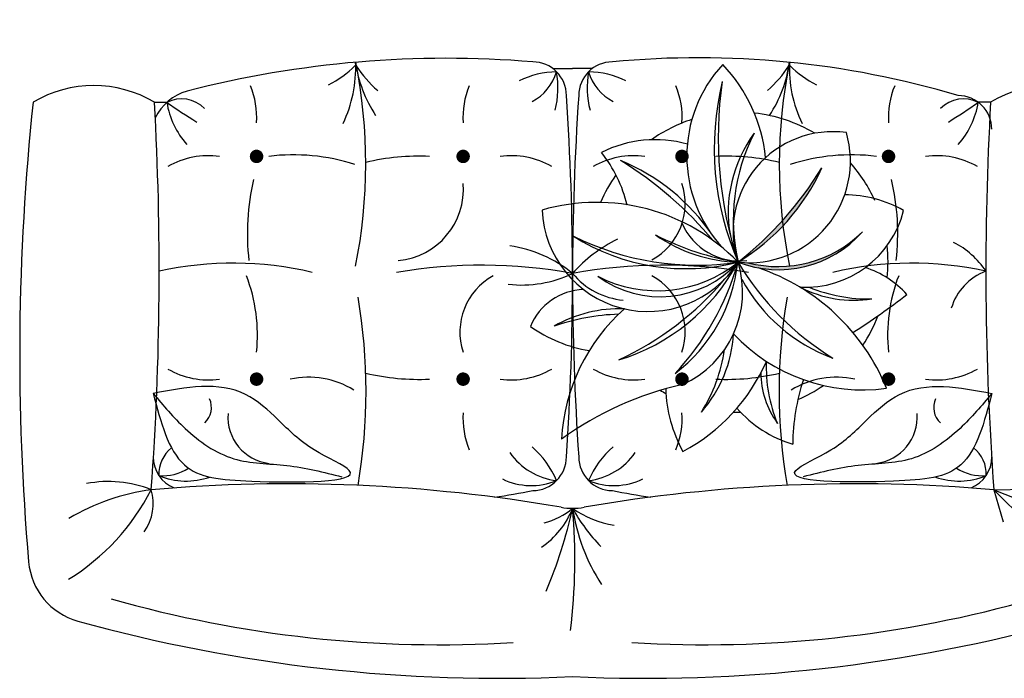
# Model space of a CAD drawing. Units: inches. Extents: x 844 to 2234, y 346 to 1084.
# Tile 25 of 93: x 1245 to 1268, y 664 to 679. Entities that reach past the tile are written whole.
import ezdxf

# ---------------------------------------------------------------- set-up
doc = ezdxf.new("R2010")
doc.units = ezdxf.units.IN
doc.header["$MEASUREMENT"] = 0
doc.layers.add('furniture', color=8, linetype='Continuous', lineweight=18)
for name, color, linetype in [('RA-AP-01$0$FURN', 3, 'Continuous'), ('RA-AP-02$0$FLPT', 30, 'Continuous'), ('ROOM-NO', 3, 'Continuous')]:
    doc.layers.add(name, color=color, linetype=linetype)

# ---------------------------------------------------------------- blocks, each defined once
blk = doc.blocks.new('A$C6E322C05')
at = {"layer": 'RA-AP-01$0$FURN'}
for p, q in [((6.391873508750865, -6.482044957760267), (6.516651486950081, -6.357266979564481)), ((6.391873508750865, -6.482044957760271), (6.43343929223883, -6.37746472106399)), ((6.391873508750866, -6.48204495776027), (6.390422568951521, -6.415535276369585)), ((6.391873508750865, -6.482044957760271), (6.439305270696451, -6.46824831830364)), ((5.817206456966433, -6.486712009544905), (5.817206456965108, -6.505053364959449)), ((5.767206456949363, -7.077520703653457), (5.767206456948565, -7.10671200954539)), ((5.767206456949363, -7.135903315437323), (5.767206456948565, -7.10671200954539)), ((5.817206456966433, -7.726712009545875), (5.817206456965108, -7.70837065413133))]:
    blk.add_line(p, q, dxfattribs=at)
at = {"layer": 'RA-AP-01$0$FURN', "const_width": 0.01}
for points in [[(5.902459393885763, -6.638129816788149, 1), (5.892459393885761, -6.638129816788122, 1)], [(6.222844373610339, -6.638129816788595, -1), (6.23284437361034, -6.638129816788595, -1)], [(5.902459393885763, -6.944444251846759, -1), (5.892459393885761, -6.944444251846785, -1)], [(6.222844373610339, -6.944444251846313, 1), (6.23284437361034, -6.944444251846313, 1)], [(5.902459393885763, -7.268979767244021, 1), (5.892459393885761, -7.268979767243994, 1)], [(6.222844373610339, -7.268979767244466, -1), (6.23284437361034, -7.268979767244466, -1)], [(5.902459393885763, -7.575294202302631, -1), (5.892459393885761, -7.575294202302657, -1)], [(6.222844373610339, -7.575294202302185, 1), (6.23284437361034, -7.575294202302185, 1)]]:
    blk.add_lwpolyline(points, format="xyb", close=True, dxfattribs=at)
at = {"layer": 'RA-AP-01$0$FURN'}
for centre, radius, start, end in [((6.192206456970573, -9.839674509409203), 3.552808610866049, 85.0473312316412, 96.0588723756579), ((5.962206456956505, -6.396712009545393), 0.1706604816468166, 148.1725534208377, 211.8274465791593), ((6.490296991311982, -6.399757455669855), 0.1, 15.49949460085664, 85.04733123164101), ((4.33669785707999, -6.99698289606033), 2.33487526667919, 357.3063521928599, 15.49949460085664), ((4.846593614069285, -6.909687157115225), 1.775196618325768, 356.4780136403396, 15.93354743557553), ((6.068281987477935, -2.019830784287151), 4.473931917517753, 266.7828902523826, 274.1477233631118), ((8.747044799885572, -6.68548500417652), 2.363941552380466, 175.0630368065897, 189.8434409139549), ((5.857266904022845, -6.534972599266733), 0.05, 90.00000000094654, 180), ((6.134026645419561, -6.595486433826224), 0.1214600988114338, 123.1053299945123, 153.7006015369794), ((6.565877894706778, -6.603111116245941), 0.5100538472773755, 167.6182489359307, 193.3122231353938), ((6.14746341585187, -6.463466129962243), 0.0853281020358404, 200.7831020638199, 253.0462459140071), ((6.367926665937501, -6.54114871013533), 0.0478550828899777, 86.575295631534, 142.6833829238214), ((6.343036863464309, -6.534972599266733), 0.05, 22.58267242460392, 89.99999999905346), ((6.302747869360707, -6.499593011892033), 0.0683206773889159, 326.6729861493449, 5.218395042636973), ((6.274768375315671, -6.53387763124781), 0.1042084262671507, 340.4828318717155, 22.86929393278168), ((5.860011614985668, -6.526983908613928), 0.0479292786975047, 152.8070868543555, 225.4025460716553), ((5.798239671935704, -6.625433523557484), 0.1218651776285568, 48.0375529564433, 81.0462320954125), ((4.904259194880517, -7.136565421857206), 1.11020813118073, 31.93286085977143, 34.66647731879807), ((6.017778833798976, -6.566879816788349), 0.1214118203512435, 150.1419074485596, 187.691663289156), ((6.107524933697323, -6.566879816788473), 0.1214118203512435, 352.3083367106845, 29.85809255128089), ((7.09459581372041, -6.919286936999045), 1.343470592134322, 163.3777289595395, 185.4806594039327), ((6.269780256940199, -6.54020363968894), 0.0310151388417235, 245.7760318513891, 317.3789451550392), ((6.284290296802319, -6.664490968717984), 0.0689028341546707, 6.419517109091462, 94.46157264568865), ((6.011601695098697, -6.976164478788355), 0.3517162425384579, 83.41248966761121, 103.1674570565571), ((6.162348040003244, -6.395238182300004), 0.2442261434243043, 248.9017070735605, 275.9923925191661), ((5.839565409091811, -6.517091257029312), 0.1212957045587361, 247.3375839744822, 273.7314750942433), ((6.197523316847625, -6.692545952238853), 0.3023568492824586, 173.0944825511667, 197.588060785551), ((6.354517986346992, -6.715077923337803), 0.1295083186917369, 167.9901339202812, 211.3796151021958), ((5.650260521516567, -6.673548227893377), 0.1579426672576338, 315.4052081938554, 333.0844958846701), ((5.765922189292775, -6.593612516654137), 0.1915923630277471, 267.5852697713958, 295.5830728418392), ((5.908792452070163, -6.03459657477793), 0.765467899454341, 258.6273206109321, 281.4174148186357), ((5.73314461686815, -6.969744817001631), 0.1863549309199891, 56.29262493376822, 82.3818003344588), ((5.679375702373212, -6.920075501166131), 0.1579426672576338, 40.38651175517922, 58.06579944599388), ((6.245858341704271, -5.977214432993086), 0.8232838708255751, 260.2449188973366, 279.7550811026635), ((6.245792934290092, -6.879444251846194), 0.3486563571350461, 166.839178360846, 182.4657575311016), ((5.879510833205829, -6.879444251846704), 0.3486563571350461, 357.5342424690579, 13.1608216393135), ((6.80739198570858, -6.9716011229856), 0.7485435294774117, 170.3094183042209, 190.3986311369044), ((5.959527339947079, -6.859074294904489), 0.0930420630931112, 293.6025128512426, 6.610683813350465), ((5.839565409091811, -7.065482811605596), 0.1212957045587361, 86.2685249057567, 112.6624160255178), ((5.967289987028921, -7.035039638983766), 0.0953802309589454, 28.80342840007747, 108.2253060204472), ((6.158013780467433, -7.035039638983501), 0.0953802309589454, 71.7746939797123, 151.196571600082), ((6.285738358404627, -7.065482811604976), 0.1212957045587361, 67.33758397464167, 93.73147509440282), ((5.08702348459791, -6.791287034316994), 1.330927509443381, 348.8964178164725, 351.3771209523497), ((6.017778833798976, -7.015694251846559), 0.1214118203512435, 172.308336710844, 209.8580925514404), ((6.107524933697323, -7.015694251846435), 0.1214118203512435, 330.1419074487191, 7.691663289315497), ((6.286338558013386, -7.045586518350251), 0.0993499474027353, 337.9047121936679, 25.63436525513283), ((6.280014948979332, -7.094901076442985), 0.0990996950214925, 6.922564260119504, 55.10883789097723), ((5.904234274973987, -7.085727051545815), 0.1323517050571434, 153.8887786398558, 178.8006589660143), ((5.999456242224805, -7.021102361717039), 0.1116589361851176, 309.9425663137084, 354.6905921774272), ((5.807266904022846, -7.047601469367252), 0.05, 180, 269.9999999990534), ((5.751472800077547, -7.013313769593298), 0.07258027258109, 286.3558526771587, 332.6774804096085), ((6.211136556040091, -6.947122539501678), 0.212288550941915, 205.9704430982785, 228.7419974602242), ((6.4323439288987, -6.955317466880212), 0.1385734111998875, 221.2288777133949, 247.0867614897648), ((6.343036863466045, -7.047601469376512), 0.05, 269.9999999989608, 359.9999999989431), ((6.304557655687245, -7.024767404076127), 0.1410608784479501, 324.4849629611242, 351.797284145529), ((6.374625390672053, -6.818147225624045), 0.2920141296149301, 278.8152064253152, 302.6921045175205), ((6.285596300104752, -6.865193601455727), 0.2760944594998999, 298.9825510110601, 313.6694461006315), ((5.795585623761384, -6.952739633017071), 0.1323517050571434, 259.6959164764198, 284.6077968025783), ((6.319376003798462, -7.10671200954539), 0.1, 350.1565590860452, 9.843440913955273), ((6.075151883811576, -3.163731520221818), 3.942980489323571, 266.1043400737264, 273.8956599242929), ((6.075151883808545, -11.04969249895812), 3.942980489412734, 86.10434007575122, 93.89565992614118), ((6.213892115887508, -7.225151532818968), 0.1854874288882049, 140.3167953258794, 172.0522897837384), ((6.80739198570858, -7.241822896105179), 0.7485435294774117, 169.6010516837189, 189.690581695779), ((5.911254573522987, -7.182496879996349), 0.1769409696162427, 353.679636560008, 25.3608296845614), ((6.496371549498975, -7.961935855380467), 0.8586827939016008, 83.03755924582121, 95.14445252709366), ((6.375720249476352, -7.220682794696101), 0.1220457486080966, 33.71356548940426, 69.04099283815023), ((6.338324584842819, -7.175279287582296), 0.1061640434993627, 14.36483859718907, 40.23030537468725), ((6.269502792941208, -7.789055933740261), 0.6986094833441214, 67.00911261779231, 77.61200156369726), ((4.336697857080025, -7.216441123030454), 2.334875266679154, 344.5005053991432, 2.69364780714023), ((5.807266904022846, -7.165822549723527), 0.05, 90.00000000094654, 180), ((6.343036863466045, -7.165822549714267), 0.05, 1.0568602e-09, 90.00000000103913), ((8.747044799885572, -7.527939014914259), 2.363941552380466, 170.156559086045, 184.9369631934102), ((5.795585623761384, -7.260684386073708), 0.1323517050571434, 75.39220319742172, 100.3040835235802), ((5.904234274973987, -7.127696967544965), 0.1323517050571434, 181.1993410339857, 206.1112213601442), ((5.751472800077547, -7.200110249497481), 0.07258027258109, 27.32251959039153, 73.64414732284132), ((6.017778833798976, -7.19772976724422), 0.1214118203512435, 150.1419074485596, 187.691663289156), ((6.107524933697323, -7.197729767244345), 0.1214118203512435, 352.3083367106845, 29.85809255128088), ((6.4323439288987, -7.25810655221026), 0.1385734111998875, 112.9132385102352, 138.7711222866051), ((6.280014948979332, -7.118522942647487), 0.0990996950214925, 304.8911621090228, 353.0774357398805), ((6.286338558013386, -7.167837500740221), 0.0993499474027353, 334.3656347448672, 22.09528780633203), ((7.290981934450236, -7.293982589837588), 1.539060359583382, 175.2233567466078, 194.4661216781742), ((5.08702348459791, -7.422136984773786), 1.330927509443381, 8.62287904765033, 11.10358218352746), ((4.846593614069285, -7.303736861975558), 1.775196618325768, 344.0664525644245, 3.521986359660393), ((6.158013780467433, -7.178384380107278), 0.0953802309589454, 208.803428399918, 288.2253060202877), ((5.839565409091811, -7.147941207485184), 0.1212957045587361, 247.3375839744822, 273.7314750942433), ((5.946346035540796, -7.374645549675604), 0.1060388135390937, 5.185910074000148, 94.80734315124221), ((6.285738358404627, -7.147941207485803), 0.1212957045587361, 266.2685249055972, 292.6624160253583), ((6.245792934290092, -7.333979767244585), 0.3486563571350461, 177.5342424688983, 193.160821639154), ((5.879510833205829, -7.333979767244075), 0.3486563571350461, 346.8391783606865, 2.465757530942165), ((5.73314461686815, -7.243679202089149), 0.1863549309199891, 277.6181996655412, 303.7073750662318), ((5.679375702373212, -7.293348517924648), 0.1579426672576338, 301.9342005540061, 319.6134882448208), ((5.908792452070163, -8.17882744431285), 0.765467899454341, 78.58258518136427, 101.3726793890678), ((6.245858341704271, -8.236209586097694), 0.8232838708255751, 80.24491889733653, 99.75508110266345), ((5.765922189292775, -7.619811502436642), 0.1915923630277471, 64.41692715816083, 92.41473022860427), ((5.650260521516567, -7.539875791197403), 0.1579426672576338, 26.91550411532996, 44.59479180614462), ((6.197523316847625, -7.520878066851927), 0.3023568492824586, 162.411939214449, 186.9055174488332), ((6.354517986346992, -7.498346095752976), 0.1295083186917369, 148.6203848978042, 192.0098660797188), ((6.565877894706778, -7.610312902844838), 0.5100538472773755, 166.6877768646062, 192.3817510640693), ((6.284290296802319, -7.548933050372795), 0.0689028341546707, 265.5384273543114, 353.5804828909086), ((5.839565409091811, -7.696332762061468), 0.1212957045587361, 86.26852490575668, 112.6624160255178), ((6.162348040003244, -7.818185836790775), 0.2442261434243043, 84.00760748083387, 111.0982929264395), ((6.011601695098697, -7.237259540302424), 0.3517162425384579, 256.8325429434429, 276.5875103323888), ((6.017778833798976, -7.646544202302431), 0.1214118203512435, 172.308336710844, 209.8580925514404), ((6.107524933697323, -7.646544202302306), 0.1214118203512435, 330.1419074487191, 7.691663289315504), ((6.269780256940199, -7.67322037940184), 0.0310151388417235, 42.62105484496073, 114.2239681486109), ((6.274768375315671, -7.679546387842969), 0.1042084262671507, 337.1307060672183, 19.51716812828453), ((5.860011614985668, -7.686440110476851), 0.0479292786975047, 134.5974539283447, 207.1929131456445), ((4.904259194880517, -7.076858597233573), 1.11020813118073, 325.333522681202, 328.0671391402286), ((5.87316911435942, -7.657653239374848), 0.0753785023123622, 196.0166452769965, 244.1254380939442), ((5.798239671935704, -7.587990495533295), 0.1218651776285568, 278.9537679045876, 311.9624470435567), ((6.302747869360707, -7.713831007198747), 0.0683206773889159, 354.781604957363, 33.32701385065516), ((6.367926665937501, -7.672275308955449), 0.0478550828899777, 217.3166170761785, 273.424704368466), ((6.343036863464309, -7.678451419824046), 0.05, 270.0000000009465, 337.4173275753961), ((6.068281987477935, -12.19359323480363), 4.473931917517753, 85.85227663688822, 93.21710974761734), ((5.966706456956126, -7.816712009545387), 0.1744999999876311, 148.9517780040469, 211.0482219959533), ((6.549562589740832, -7.794613830093475), 0.1698955038956699, 158.1487616198804, 191.122156864055), ((6.412319729336772, -7.798818772412041), 0.0704710051510922, 53.58735038429053, 106.8661365794674), ((6.713110001951175, -7.687961227420911), 0.3241573581843151, 187.6973649013944, 210.7014325157311), ((6.237117433414106, -8.032110101276656), 0.3382138395168437, 31.74362916573515, 62.76966729059727), ((6.49029699131198, -7.813666563420925), 0.1, 274.9526687683584, 344.500505399143), ((6.192206456970577, -4.373749509681577), 3.552808610866049, 263.941127624342, 274.9526687683587)]:
    blk.add_arc(centre, radius, start, end, dxfattribs=at)
for points, knots in [([(6.249068123947751, -6.484897777661085), (6.239897409094627, -6.533353418276971), (6.226611264288107, -6.603553906267942), (6.290696373977354, -6.673990528916563), (6.332121563214334, -6.713363084361603), (6.381789098403072, -6.831232979612737), (6.381738454094183, -6.629656072516828), (6.370771929626907, -6.516634365426866), (6.291185937762818, -6.495880800642047), (6.249068123947751, -6.484897777661087)], [0, 0, 0, 0, 0.1367586589314792, 0.1981301758052368, 0.2677729570689282, 0.3281194902553322, 0.4737578340741565, 0.5765194025309516, 0.6920332287422236, 0.6920332287422236, 0.6920332287422236, 0.6920332287422236]), ([(6.249068123947751, -6.484897777661087), (6.266851662635476, -6.499857019491296), (6.306238891621481, -6.532988956490432), (6.353826300430336, -6.600137645661404), (6.352465874908733, -6.685122080531377), (6.365878290565239, -6.737689715716581), (6.372748706337224, -6.764617117843226)], [0, 0, 0, 0, 0.070018540671015, 0.1550780383534498, 0.2344491945777043, 0.3178048737568289, 0.3178048737568289, 0.3178048737568289, 0.3178048737568289]), ([(6.249068123947751, -7.728526241429694), (6.239897409094627, -7.680070600813808), (6.226611264288107, -7.609870112822835), (6.290696373977354, -7.539433490174218), (6.332121563214334, -7.500060934729178), (6.381789098403072, -7.382191039478041), (6.381738454094183, -7.583767946573952), (6.370771929626907, -7.696789653663914), (6.291185937762818, -7.717543218448732), (6.249068123947751, -7.728526241429692)], [0, 0, 0, 0, 0.1367586589314792, 0.1981301758052368, 0.2677729570689282, 0.3281194902553322, 0.4737578340741565, 0.5765194025309516, 0.6920332287422236, 0.6920332287422236, 0.6920332287422236, 0.6920332287422236]), ([(6.249068123947751, -7.728526241429692), (6.266851662635476, -7.713566999599485), (6.306238891621481, -7.680435062600349), (6.353826300430336, -7.613286373429378), (6.352465874908733, -7.528301938559401), (6.365878290565239, -7.475734303374198), (6.372748706337224, -7.448806901247554)], [0, 0, 0, 0, 0.070018540671015, 0.1550780383534498, 0.2344491945777043, 0.3178048737568289, 0.3178048737568289, 0.3178048737568289, 0.3178048737568289])]:
    blk.add_open_spline(points, degree=3, knots=knots, dxfattribs=at)
blk = doc.blocks.new('A$C78016F37')
at = {"layer": 'RA-AP-02$0$FLPT'}
for points in [[(8.585816203069419, -6.02390819987247, -0.263770389754008), (8.460672408962632, -5.900531828839305, -0.0241291823863587), (8.454072418949808, -5.887595694471202, 2.53684562776e-05), (8.45404743172537, -5.887630207283394, 0.3135010205465867)], [(8.6375288720004, -5.923949758415821, -0.0887687358956854), (8.454121692088984, -5.887527659105068, 7.7903089823e-06), (8.45411401635844, -5.887538255716633, 0.1521261679004899)]]:
    blk.add_hatch(color=256, dxfattribs=at).paths.add_polyline_path(points)
at = {"layer": 'RA-AP-01$0$FURN'}
for centre, radius, start, end in [((8.676215054199671, -5.667660989702041), 0.3125591380039201, 178.1117989109854, 224.6938723266582), ((8.77416640415315, -5.62926868308301), 0.4113013577889528, 183.916601998098, 218.889069239545), ((8.454024671827373, -5.887489670112504), 0.2224048992971994, 84.85146405771819, 96.8968759960221), ((7.926806489084671, -5.648344237112944), 0.5693232143741963, 340.3683676450975, 358.6332230039188), ((8.195746570571197, -5.703566525505195), 0.3030929277970076, 334.410018118324, 8.056842366720524), ((8.454024671827373, -5.887489670112504), 0.2224048992971994, 48.29632106119188, 65.66234443375417), ((8.028579057188336, -5.942548842808446), 0.3176725093823991, 32.12276904396682, 49.65676958807643), ((8.138392155386812, -5.868774225710474), 0.1937166188785145, 28.24647600965292, 60.3482035660113), ((8.485489110864293, -5.735116799889917), 0.1555876039528135, 173.9896977683083, 258.3326220930856), ((8.521327457039675, -5.708924385009453), 0.1908277389198635, 182.9741757068071, 249.3481441545862), ((8.654249619708994, -5.778555799161595), 0.2279399438329033, 175.7401143551485, 208.5487298435666), ((8.841321835932057, -5.738299260526738), 0.4150383977849519, 183.2217031044116, 201.067141094303), ((8.454024671827373, -5.887489670112504), 0.2224048992971994, 359.5998786150253, 24.14255533511359), ((8.442163868805496, -5.589503946884691), 0.2981456377964393, 227.2393731923049, 272.0875214538299), ((8.499731284894388, -5.433816546692462), 0.4559697329776795, 235.2365058162176, 260.2774785796924), ((8.610008543493892, -6.006599373458567), 0.1961871509349957, 83.84242350983102, 130.6121505715144), ((8.645911592327788, -6.090477518425219), 0.27932894017942, 93.04938662579335, 133.3896949469156), ((8.564547574985227, -5.985184712735347), 0.1475114689626245, 22.41040215178937, 138.5254141817128), ((8.454024671827373, -5.887489670112504), 0.2224048992971994, 179.1222698891959, 181.6416201752811), ((8.343226438185093, -5.786283478281637), 0.1500631261941314, 234.481997856841, 317.590554229248), ((8.35533458686642, -5.671200371653297), 0.2372928460263133, 247.4602721701189, 294.3106346998744), ((8.353310301606033, -5.50080131865886), 0.3995888706145134, 257.1400840392136, 284.5985568218482), ((8.820839898988444, -6.089372712149781), 0.4186128907603021, 151.1845644972185, 178.7925181665867), ((8.647592804319403, -5.39327801538501), 0.5307671632505924, 248.6111860886518, 268.9135435570199), ((8.591324349397098, -5.825721750746069), 0.1505539017216363, 204.2218678925879, 316.713948440902), ((8.60427433017431, -5.61130057980146), 0.3144127437625546, 241.4533621372112, 276.0713675084609), ((8.617925276426345, -5.861018191689067), 0.1660245384207697, 189.1745772070899, 258.8487542743241), ((8.650970463531563, -6.036034461900849), 0.252604074752176, 148.7548044074418, 190.1503402437527), ((8.632043935228618, -5.851861780578565), 0.1781487401371014, 195.8547118906642, 254.9602254039967), ((8.27103219642381, -5.762377687346963), 0.1942058542978326, 259.1738264472347, 296.9361074578899), ((8.242487148295718, -5.713440208635033), 0.2398180026482373, 268.1044384936476, 291.9165885710061), ((8.454024671827373, -5.887489670112504), 0.2224048992971994, 324.5751954876287, 341.8360454133948), ((8.643418645519843, -5.97565241718072), 0.1753165964770544, 183.2000241261284, 219.1319783506275), ((8.454024671827373, -5.887489670112504), 0.2224048992971994, 208.6999597596628, 211.2898901048327), ((8.447576280134497, -6.186493140077375), 0.2128537218708566, 117.7922244992203, 143.1680179163233), ((8.391080266506174, -6.106601067273632), 0.1233275614230441, 120.0065551025349, 157.0200898875673), ((8.702436309821351, -5.965526387054176), 0.2293777808440535, 187.970132899875, 211.770006950379), ((8.454024671827373, -5.887489670112504), 0.2224048992971994, 233.8814212202215, 245.0364073377333), ((8.454024671827373, -5.887489670112504), 0.2224048992971994, 294.3332330132876, 306.7022905924929), ((8.454024671827373, -5.887489670112504), 0.2224048992971994, 266.6746775461067, 279.4836973606225)]:
    blk.add_arc(centre, radius, start, end, dxfattribs=at)
at = {"layer": 'RA-AP-02$0$FLPT'}
blk.add_lwpolyline([(8.373681407360612, -5.597603282219753, 0.7334826821515817), (8.454024671827373, -5.887489670112506, 0.2766279680881699), (8.373681407360612, -5.597603282219752, 1.3559471233864)], format="xyb", dxfattribs=at)
for centre, radius, start, end in [((8.307234168263015, -5.560224752275053), 0.1974581866646199, 313.6950443365965, 339.1517930721081), ((8.39717548070647, -5.778250590985688), 0.1754354389711152, 14.56900959352841, 57.37320031926483), ((8.423880035729836, -5.687934118592295), 0.2086915776254087, 175.0742803806306, 201.2122531761669), ((8.228139151249446, -5.75774524127399), 0.0885717136803359, 32.28640253436571, 97.90409188948885), ((8.433135668112254, -6.051756800567661), 0.1760533926534347, 161.4400574260173, 193.8427700955681), ((8.41746442128814, -6.364284642428606), 0.3118134108627832, 101.9980156162763, 119.8647524560376), ((8.395985399479063, -6.084837299933293), 0.1497734353479364, 343.3485825573843, 11.74756506179821), ((8.942045887600607, -5.120169675385827), 1.085029101271162, 243.0359441902965, 248.2214525024466)]:
    blk.add_arc(centre, radius, start, end, dxfattribs=at)
at = {"layer": 'ROOM-NO'}
for centre, radius, start, end in [((8.65235909715731, -5.915275987506324), 0.2002713751519826, 77.61332513631854, 163.1649854687259), ((8.46944987509335, -5.65497750757116), 0.2349499976215632, 306.2836330402241, 344.0182681768919), ((8.897731643814414, -6.279909663508004), 0.5923422390868573, 112.2662452820337, 138.5100534847894), ((8.794175340646271, -6.133856003178959), 0.4198977696908007, 106.7322927724504, 144.0984247900076), ((8.22288024947718, -6.040653787747125), 0.2772850355038946, 71.89678357893693, 117.3860017964977), ((7.898132843717886, -6.242790504972724), 0.48979813475044, 43.05187184217114, 66.25811984072557), ((8.347851773195234, -6.064576052783105), 0.2064758371609359, 122.2147792747386, 149.2270256684313), ((8.154124515379644, -5.981454547332234), 0.314276155615234, 322.6594768637323, 11.71644421186061), ((8.609526443069848, -6.010438452646774), 0.261483616160276, 163.3494523104177, 218.1824089018609), ((8.3154997513214, -5.724318991124441), 0.2758350084868725, 238.2734303421065, 276.8355613505966), ((8.602078464955955, -5.915823919619132), 0.1507406891149966, 207.5045866236536, 286.2267783265413), ((8.468611314717652, -6.062483436674201), 0.1756006505860901, 0.6277371554985871, 30.43990742705027)]:
    blk.add_arc(centre, radius, start, end, dxfattribs=at)
blk = doc.blocks.new('A$C5D2F253E')
at = {"layer": 'RA-AP-01$0$FURN', "xscale": -1}
blk.add_blockref('A$C6E322C05', (4.620200485489021, 7.961130550668883), dxfattribs=at)
at = {"layer": 'RA-AP-02$0$FLPT', "xscale": -1, "rotation": 210.3787734063952}
blk.add_blockref('A$C78016F37', (-5.749960471669055, -8.254610923396115), dxfattribs=at)

msp = doc.modelspace()

# ---------------------------------------------------------------- block references
at = {"layer": 'furniture', "xscale": -15.94108302203742, "yscale": 15.94108302203742, "zscale": 15.94108302203742, "rotation": 270}
msp.add_blockref('A$C5D2F253E', (1244.08405109492, 696.2584716700112), dxfattribs=at)

doc.saveas('drawing.dxf')
